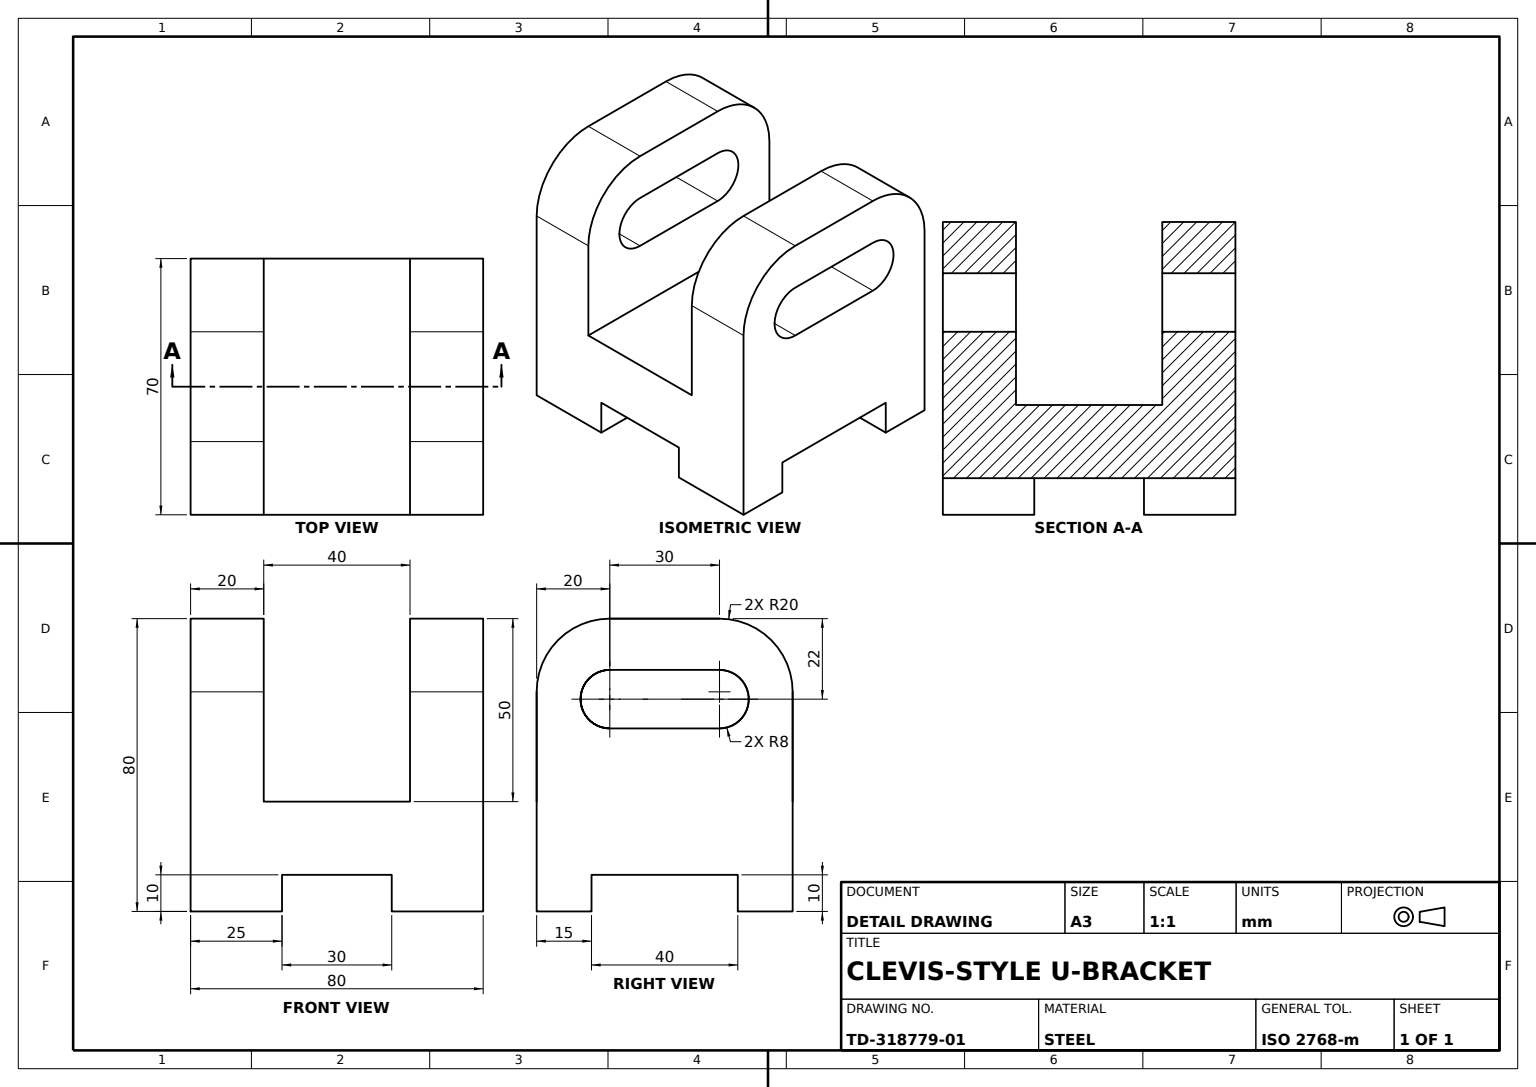
from build123d import *

# Parameters (mm, degrees)
BASE_BLOCK_PROFILE_80X80_W  = 80
BASE_BLOCK_PROFILE_80X80_H  = 80
BASE_BLOCK_80X80X70_DEPTH   = 35
NOTCH_CUT_20X20_DEPTH       = 91
NOTCH_CUT_20X20_DEPTH_BACK  = 91
NOTCH_PROFILE_20X20_W       = 40
NOTCH_PROFILE_20X20_H       = 50
NOTCH_CUT_25X25_DEPTH       = 91
NOTCH_CUT_25X25_DEPTH_BACK  = 91
NOTCH_PROFILE_25X25_W       = 30
NOTCH_PROFILE_25X25_H       = 10
POCKET_CUT_40X15_DEPTH      = 97.046863561
POCKET_CUT_40X15_DEPTH_BACK = 97.046863561
POCKET_PROFILE_40X15_W      = 40
POCKET_PROFILE_40X15_H      = 10
UPRIGHT_SLOT_CUT_DEPTH      = 97.046863561
UPRIGHT_SLOT_CUT_DEPTH_BACK = 97.046863561
UPRIGHT_TOP_FILLETS_R20_R   = 20


with BuildPart() as part:
    # Base Block Profile 80x80 → Base Block 80x80x70 (new, symmetric)
    with BuildSketch(Plane(origin=(0, 0, 0), x_dir=(0, 0, -1), z_dir=(1, 0, 0))):
        Rectangle(BASE_BLOCK_PROFILE_80X80_W, BASE_BLOCK_PROFILE_80X80_H)
    extrude(amount=BASE_BLOCK_80X80X70_DEPTH, both=True)

    # Notch Profile 20x20 → Notch Cut 20x20 (cut, two sides: drawn at the far end of the back side and taken through both)
    with BuildSketch(Plane(origin=(35, 0, 0), x_dir=(0, 0, -1), z_dir=(1, 0, 0)).offset(-NOTCH_CUT_20X20_DEPTH_BACK)):
        with Locations((0, 15)):
            Rectangle(NOTCH_PROFILE_20X20_W, NOTCH_PROFILE_20X20_H)
    extrude(amount=NOTCH_CUT_20X20_DEPTH + NOTCH_CUT_20X20_DEPTH_BACK, mode=Mode.SUBTRACT)

    # Notch Profile 25x25 → Notch Cut 25x25 (cut, two sides: drawn at the far end of the back side and taken through both)
    with BuildSketch(Plane(origin=(35, 0, 0), x_dir=(0, 0, -1), z_dir=(1, 0, 0)).offset(-NOTCH_CUT_25X25_DEPTH_BACK)):
        with Locations((0, -35)):
            Rectangle(NOTCH_PROFILE_25X25_W, NOTCH_PROFILE_25X25_H)
    extrude(amount=NOTCH_CUT_25X25_DEPTH + NOTCH_CUT_25X25_DEPTH_BACK, mode=Mode.SUBTRACT)

    # Pocket Profile 40x15 → Pocket Cut 40x15 (cut, two sides: drawn at the far end of the back side and taken through both)
    with BuildSketch(Plane.XY.offset(40).offset(-POCKET_CUT_40X15_DEPTH_BACK)):
        with Locations((0, -35)):
            Rectangle(POCKET_PROFILE_40X15_W, POCKET_PROFILE_40X15_H)
    extrude(amount=POCKET_CUT_40X15_DEPTH + POCKET_CUT_40X15_DEPTH_BACK, mode=Mode.SUBTRACT)

    # Upright Slot Profile → Upright Slot Cut (cut, two sides: drawn at the far end of the back side and taken through both)
    with BuildSketch(Plane.XY.offset(40).offset(-UPRIGHT_SLOT_CUT_DEPTH_BACK)):
        with BuildLine():
            Line((-15, 26), (15, 26))
            ThreePointArc((15, 26), (23, 18), (15, 10))
            Line((15, 10), (-15, 10))
            ThreePointArc((-15, 10), (-23, 18), (-15, 26))
        make_face()
    extrude(amount=UPRIGHT_SLOT_CUT_DEPTH + UPRIGHT_SLOT_CUT_DEPTH_BACK, mode=Mode.SUBTRACT)

    # Upright Top Fillets R20
    upright_top_fillets_r20_edges = [part.edges().sort_by_distance(p)[0] for p in [
        (-35, 40, 30),
        (35, 40, 30),
        (-35, 40, -30),
        (35, 40, -30),
    ]]
    fillet(upright_top_fillets_r20_edges, radius=UPRIGHT_TOP_FILLETS_R20_R)


solid = part.part
